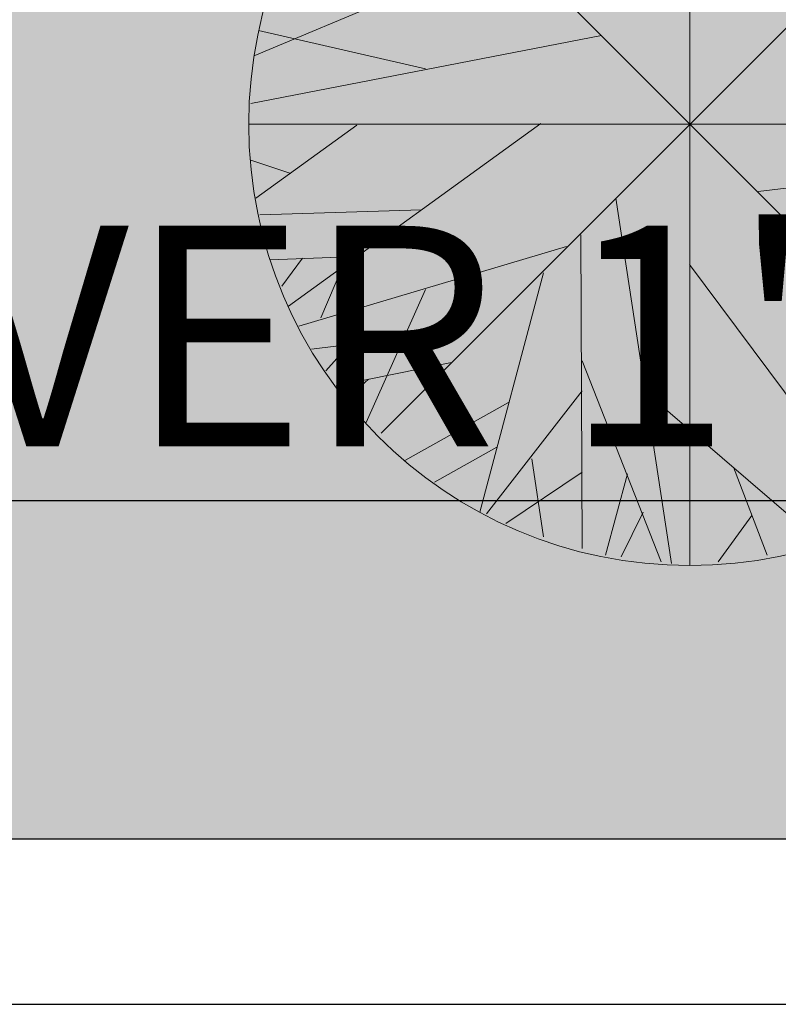
# Model space of a CAD drawing. Units: inches. Extents: x 459864 to 460310, y 324185 to 324787.
# Tile 56 of 112: x 460169 to 460189, y 324195 to 324222. Entities that reach past the tile are written whole.
import ezdxf

# ---------------------------------------------------------------- set-up
doc = ezdxf.new("R2010")
doc.units = ezdxf.units.IN
for name, color, linetype, lineweight in [('A-ANNO-DIMS', 2, 'Continuous', 18), ('C-PROP', 7, 'Continuous', 30), ('L-PLNT', 3, 'Continuous', 13), ('L-SITE-PATT', 252, 'Continuous', 13)]:
    doc.layers.add(name, color=color, linetype=linetype, lineweight=lineweight)
doc.styles.get("Standard").update_dxf_attribs({"font": 'arial.ttf'})
doc.dimstyles.new('ISO-25', dxfattribs={"dimtxt": 6, "dimasz": 2.5, "dimexe": 1.25, "dimexo": 0.625, "dimtad": 1, "dimdec": 1, "dimlunit": 3, "dimtxsty": 'Standard', "dimcen": 2.5, "dimadec": 0, "dimazin": 0, "dimtfac": 1, "dimtdec": 1, "dimtmove": 0, "dimatfit": 3, "dimfxl": 1, "dimarcsym": 0})

# ---------------------------------------------------------------- blocks, each defined once
blk = doc.blocks.new('Tree - deciduous plan')
for p, q in [((0, 59.9996), (0, -60)), ((42, 42), (-42, -42)), ((42, -42), (-42, 42)), ((-32.2571, 20.6333), (-59.1937, 9.348)), ((-59.7219, 2.8025), (-12.0106, 12.0565)), ((-58.6656, 12.7336), (-35.9543, 7.5424)), ((-54.6162, -24.7335), (-20.2853, 0.0941)), ((-60, 0), (60, 0)), ((-45.2853, -0.1316), (-59.0177, -10.0627)), ((9.2922, -9.1598), (59.6443, -2.8401)), ((-59.7219, -4.8714), (-54.2641, -6.6771)), ((-10.074, -10.0627), (-2.5036, -59.7178)), ((-58.4895, -12.3197), (-36.4825, -11.6426)), ((-14.8275, -15.0282), (-14.6515, -57.6865)), ((-53.2078, -27.442), (-16.7641, -16.6081)), ((-57.081, -18.4138), (-45.2853, -17.9624)), ((-52.6797, -18.188), (-55.4966, -22.0251)), ((-47.2219, -19.3166), (-50.2148, -26.3135)), ((-0.0388, -19.0909), (25.8415, -53.8495)), ((-19.9331, -20.2194), (-28.5599, -52.721)), ((-35.9543, -22.4765), (-44.0529, -40.5329)), ((-38.9472, -29.0219), (-51.4472, -30.6018)), ((-46.5177, -30.1504), (-49.5106, -33.536)), ((-32.4331, -32.4075), (-48.1021, -35.5674)), ((-14.6515, -32.1818), (-3.912, -59.4922)), ((-43.7008, -34.6645), (-46.6937, -37.373)), ((-14.6515, -36.2445), (-27.6797, -52.9467)), ((-6.2008, -36.2445), (17.919, -57.0094)), ((-24.6867, -37.8244), (-38.7712, -45.7241)), ((-26.2712, -43.9185), (-34.7219, -48.6583)), ((-21.5177, -45.4984), (-19.9331, -56.1065)), ((5.9471, -46.6269), (10.5246, -58.5893)), ((-14.6515, -47.3041), (-25.0388, -54.3009)), ((-8.4895, -47.5298), (-11.4825, -58.5893)), ((-6.3768, -52.721), (-9.3698, -58.815)), ((8.4119, -53.1724), (3.8344, -59.4922))]:
    blk.add_line(p, q)
blk.add_circle((0, 0), 60)
blk = doc.blocks.new('*D34')
at = {"layer": 'A-ANNO-DIMS', "color": 0, "lineweight": -2, "transparency": 16777216}
for p, q in [((460132.814, 324211.063), (460132.814, 324207.434)), ((460152.838, 324211.063), (460152.838, 324207.434)), ((460135.314, 324208.684), (460150.338, 324208.684)), ((460152.838, 324208.684), (460202.984, 324208.684))]:
    blk.add_line(p, q, dxfattribs=at)
at = {"layer": 'A-ANNO-DIMS', "color": 0, "transparency": 16777216}
for points in [[(460135.314, 324209.101), (460135.314, 324208.268), (460132.814, 324208.684)], [(460150.338, 324209.101), (460150.338, 324208.268), (460152.838, 324208.684)]]:
    blk.add_solid(points, dxfattribs=at)
at = {"layer": 'Defpoints', "color": 0, "transparency": 16777216}
for p in [(460132.814, 324211.688), (460152.838, 324211.688), (460152.838, 324208.684)]:
    blk.add_point(p, dxfattribs=at)
at = {"layer": 'A-ANNO-DIMS', "color": 0, "transparency": 16777216, "insert": (460179.161, 324212.373), "char_height": 6, "attachment_point": 5}
blk.add_mtext('PAVER 1\'-8"', dxfattribs=at)

msp = doc.modelspace()

# ---------------------------------------------------------------- hatches: boundary and pattern name
at = {"layer": 'L-SITE-PATT'}
h = msp.add_hatch(dxfattribs=at)
h.set_pattern_fill('DOTS', color=256)
h.paths.add_polyline_path([(460269.804, 324283.483), (460247.115, 324283.483), (460121.929, 324283.483), (460121.929, 324252.473), (460117.429, 324252.473), (460110.124, 324252.473), (460110.124, 324243.287), (460080.83, 324243.287), (460080.83, 324252.473), (460061.115, 324252.473), (460061.115, 324251.882), (460077.909, 324251.882), (460077.909, 324199.483), (460080.83, 324199.483), (460080.83, 324207.553), (460110.124, 324207.553), (460110.124, 324199.483), (460110.813, 324199.483), (460262.115, 324199.483), (460269.804, 324199.483)], flags=17)
edge = h.paths.add_edge_path(flags=0)
edge.add_ellipse((460222.59, 324263.813), major_axis=(-8.485, 8.485), ratio=1, start_angle=405, end_angle=495, ccw=False)
edge.add_line((460214.821, 324254.66), (460214.832, 324254.666))
edge.add_ellipse((460222.59, 324263.813), major_axis=(-8.485, 8.485), ratio=1, start_angle=405, end_angle=495, ccw=False)
edge.add_line((460210.759, 324261.781), (460210.768, 324261.787))
edge.add_ellipse((460222.59, 324263.813), major_axis=(-8.485, 8.485), ratio=1, start_angle=405, end_angle=495, ccw=False)
edge.add_ellipse((460222.59, 324263.813), major_axis=(-8.485, 8.485), ratio=1, start_angle=392.754, end_angle=405, ccw=False)
edge.add_ellipse((460222.59, 324263.813), major_axis=(-8.485, 8.485), ratio=1, start_angle=380.9347, end_angle=392.754, ccw=False)
edge.add_line((460211.337, 324267.985), (460211.34, 324267.985))
edge.add_ellipse((460222.59, 324263.813), major_axis=(-8.485, 8.485), ratio=1, start_angle=380.9347, end_angle=392.754, ccw=False)
edge.add_ellipse((460222.59, 324263.813), major_axis=(-8.485, 8.485), ratio=1, start_angle=347.9015, end_angle=380.9347, ccw=False)
edge.add_ellipse((460222.59, 324263.813), major_axis=(-8.485, 8.485), ratio=1, start_angle=327.0619, end_angle=347.9015, ccw=False)
edge.add_ellipse((460222.59, 324263.813), major_axis=(-8.485, 8.485), ratio=1, start_angle=278.3246, end_angle=327.0619, ccw=False)
edge.add_line((460225.158, 324275.536), (460225.158, 324275.535))
edge.add_ellipse((460222.59, 324263.813), major_axis=(-8.485, 8.485), ratio=1, start_angle=278.3246, end_angle=327.0619, ccw=False)
edge.add_ellipse((460222.59, 324263.813), major_axis=(-8.485, 8.485), ratio=1, start_angle=260.6436, end_angle=278.3246, ccw=False)
edge.add_ellipse((460222.59, 324263.813), major_axis=(-8.485, 8.485), ratio=1, start_angle=225, end_angle=260.6436, ccw=False)
edge.add_line((460234.509, 324265.243), (460234.501, 324265.239))
edge.add_ellipse((460222.59, 324263.813), major_axis=(-8.485, 8.485), ratio=1, start_angle=225, end_angle=260.6436, ccw=False)
edge.add_ellipse((460222.59, 324263.813), major_axis=(-8.485, 8.485), ratio=1, start_angle=495, end_angle=585, ccw=False)
edge.add_line((460234.437, 324261.861), (460234.424, 324261.858))
edge.add_ellipse((460222.59, 324263.813), major_axis=(-8.485, 8.485), ratio=1, start_angle=495, end_angle=585, ccw=False)
edge.add_line((460227.95, 324253.067), (460227.946, 324253.083))
edge.add_ellipse((460222.59, 324263.813), major_axis=(-8.485, 8.485), ratio=1, start_angle=495, end_angle=585, ccw=False)
edge.add_line((460226.223, 324252.369), (460226.211, 324252.38))
edge.add_ellipse((460222.59, 324263.813), major_axis=(-8.485, 8.485), ratio=1, start_angle=495, end_angle=585, ccw=False)
h.paths.add_polyline_path([(460219.651, 324254.347), (460218.461, 324253.545), (460218.275, 324254.789), (460219.642, 324256.542), (460219.625, 324260.848), (460216.11, 324257.333), (460214.35, 324256.978), (460215.416, 324259.356), (460212.524, 324258.496), (460213.137, 324259.93), (460218.507, 324263.813), (460222.59, 324263.813), (460222.59, 324267.807), (460218.176, 324272.212), (460219.026, 324274.639), (460222.59, 324272.811), (460222.59, 324275.423), (460223.057, 324274.825), (460222.675, 324273.492), (460225.912, 324267.135), (460219.625, 324260.848)], flags=0)
edge = h.paths.add_edge_path(flags=0)
edge.add_ellipse((460194.576, 324264.046), major_axis=(-8.485, 8.485), ratio=1, start_angle=495, end_angle=585, ccw=False)
edge.add_line((460199.936, 324253.3), (460199.932, 324253.316))
edge.add_ellipse((460194.576, 324264.046), major_axis=(-8.485, 8.485), ratio=1, start_angle=495, end_angle=585, ccw=False)
edge.add_line((460198.208, 324252.603), (460198.196, 324252.613))
edge.add_ellipse((460194.576, 324264.046), major_axis=(-8.485, 8.485), ratio=1, start_angle=495, end_angle=585, ccw=False)
edge.add_ellipse((460194.576, 324264.046), major_axis=(-8.485, 8.485), ratio=1, start_angle=405, end_angle=495, ccw=False)
edge.add_line((460186.806, 324254.893), (460186.817, 324254.899))
edge.add_ellipse((460194.576, 324264.046), major_axis=(-8.485, 8.485), ratio=1, start_angle=405, end_angle=495, ccw=False)
edge.add_line((460182.744, 324262.014), (460182.753, 324262.02))
edge.add_ellipse((460194.576, 324264.046), major_axis=(-8.485, 8.485), ratio=1, start_angle=405, end_angle=495, ccw=False)
edge.add_ellipse((460194.576, 324264.046), major_axis=(-8.485, 8.485), ratio=1, start_angle=392.754, end_angle=405, ccw=False)
edge.add_ellipse((460194.576, 324264.046), major_axis=(-8.485, 8.485), ratio=1, start_angle=380.9347, end_angle=392.754, ccw=False)
edge.add_line((460183.323, 324268.218), (460183.326, 324268.218))
edge.add_ellipse((460194.576, 324264.046), major_axis=(-8.485, 8.485), ratio=1, start_angle=380.9347, end_angle=392.754, ccw=False)
edge.add_ellipse((460194.576, 324264.046), major_axis=(-8.485, 8.485), ratio=1, start_angle=347.9015, end_angle=380.9347, ccw=False)
edge.add_ellipse((460194.576, 324264.046), major_axis=(-8.485, 8.485), ratio=1, start_angle=327.0619, end_angle=347.9015, ccw=False)
edge.add_ellipse((460194.576, 324264.046), major_axis=(-8.485, 8.485), ratio=1, start_angle=278.3246, end_angle=327.0619, ccw=False)
edge.add_line((460197.144, 324275.769), (460197.143, 324275.768))
edge.add_ellipse((460194.576, 324264.046), major_axis=(-8.485, 8.485), ratio=1, start_angle=278.3246, end_angle=327.0619, ccw=False)
edge.add_ellipse((460194.576, 324264.046), major_axis=(-8.485, 8.485), ratio=1, start_angle=260.6436, end_angle=278.3246, ccw=False)
edge.add_ellipse((460194.576, 324264.046), major_axis=(-8.485, 8.485), ratio=1, start_angle=225, end_angle=260.6436, ccw=False)
edge.add_line((460206.494, 324265.476), (460206.487, 324265.473))
edge.add_ellipse((460194.576, 324264.046), major_axis=(-8.485, 8.485), ratio=1, start_angle=225, end_angle=260.6436, ccw=False)
edge.add_ellipse((460194.576, 324264.046), major_axis=(-8.485, 8.485), ratio=1, start_angle=495, end_angle=585, ccw=False)
edge.add_line((460206.422, 324262.094), (460206.409, 324262.091))
h.paths.add_polyline_path([(460191.61, 324261.081), (460191.637, 324254.58), (460190.447, 324253.778), (460190.261, 324255.023), (460191.628, 324256.775), (460191.61, 324261.081), (460188.096, 324257.566), (460186.335, 324257.211), (460187.402, 324259.589), (460184.509, 324258.729), (460185.123, 324260.163), (460190.493, 324264.046), (460194.576, 324264.046), (460194.576, 324268.04), (460190.161, 324272.446), (460191.011, 324274.872), (460194.576, 324273.044), (460194.576, 324275.657), (460195.043, 324275.058), (460194.661, 324273.725), (460197.897, 324267.368)], flags=0)
edge = h.paths.add_edge_path(flags=0)
edge.add_ellipse((460252.912, 324263.578), major_axis=(-8.485, 8.485), ratio=1, start_angle=405, end_angle=495, ccw=False)
edge.add_line((460241.081, 324261.545), (460241.089, 324261.551))
edge.add_ellipse((460252.912, 324263.578), major_axis=(-8.485, 8.485), ratio=1, start_angle=405, end_angle=495, ccw=False)
edge.add_ellipse((460252.912, 324263.578), major_axis=(-8.485, 8.485), ratio=1, start_angle=392.754, end_angle=405, ccw=False)
edge.add_ellipse((460252.912, 324263.578), major_axis=(-8.485, 8.485), ratio=1, start_angle=380.9347, end_angle=392.754, ccw=False)
edge.add_line((460241.659, 324267.749), (460241.662, 324267.749))
edge.add_ellipse((460252.912, 324263.578), major_axis=(-8.485, 8.485), ratio=1, start_angle=380.9347, end_angle=392.754, ccw=False)
edge.add_ellipse((460252.912, 324263.578), major_axis=(-8.485, 8.485), ratio=1, start_angle=347.9015, end_angle=380.9347, ccw=False)
edge.add_ellipse((460252.912, 324263.578), major_axis=(-8.485, 8.485), ratio=1, start_angle=327.0619, end_angle=347.9015, ccw=False)
edge.add_ellipse((460252.912, 324263.578), major_axis=(-8.485, 8.485), ratio=1, start_angle=278.3246, end_angle=327.0619, ccw=False)
edge.add_line((460255.48, 324275.3), (460255.479, 324275.299))
edge.add_ellipse((460252.912, 324263.578), major_axis=(-8.485, 8.485), ratio=1, start_angle=278.3246, end_angle=327.0619, ccw=False)
edge.add_ellipse((460252.912, 324263.578), major_axis=(-8.485, 8.485), ratio=1, start_angle=260.6436, end_angle=278.3246, ccw=False)
edge.add_ellipse((460252.912, 324263.578), major_axis=(-8.485, 8.485), ratio=1, start_angle=225, end_angle=260.6436, ccw=False)
edge.add_line((460264.83, 324265.007), (460264.823, 324265.004))
edge.add_ellipse((460252.912, 324263.578), major_axis=(-8.485, 8.485), ratio=1, start_angle=225, end_angle=260.6436, ccw=False)
edge.add_ellipse((460252.912, 324263.578), major_axis=(-8.485, 8.485), ratio=1, start_angle=495, end_angle=585, ccw=False)
edge.add_line((460264.758, 324261.626), (460264.745, 324261.622))
edge.add_ellipse((460252.912, 324263.578), major_axis=(-8.485, 8.485), ratio=1, start_angle=495, end_angle=585, ccw=False)
edge.add_line((460258.272, 324252.832), (460258.268, 324252.848))
edge.add_ellipse((460252.912, 324263.578), major_axis=(-8.485, 8.485), ratio=1, start_angle=495, end_angle=585, ccw=False)
edge.add_line((460256.545, 324252.134), (460256.533, 324252.144))
edge.add_ellipse((460252.912, 324263.578), major_axis=(-8.485, 8.485), ratio=1, start_angle=495, end_angle=585, ccw=False)
edge.add_ellipse((460252.912, 324263.578), major_axis=(-8.485, 8.485), ratio=1, start_angle=405, end_angle=495, ccw=False)
edge.add_line((460245.143, 324254.424), (460245.153, 324254.43))
h.paths.add_polyline_path([(460244.672, 324256.742), (460245.738, 324259.12), (460242.846, 324258.26), (460243.459, 324259.694), (460248.829, 324263.578), (460252.912, 324263.578), (460252.912, 324267.571), (460248.497, 324271.977), (460249.348, 324274.403), (460252.912, 324272.576), (460252.912, 324275.188), (460253.379, 324274.589), (460252.997, 324273.257), (460256.233, 324266.899), (460249.946, 324260.612), (460249.973, 324254.111), (460248.783, 324253.309), (460248.597, 324254.554), (460249.964, 324256.306), (460249.946, 324260.612), (460246.432, 324257.097)], flags=0)
edge = h.paths.add_edge_path(flags=0)
edge.add_ellipse((460167.439, 324262.833), major_axis=(-8.485, 8.485), ratio=1, start_angle=495, end_angle=585, ccw=False)
edge.add_line((460172.799, 324252.087), (460172.795, 324252.103))
edge.add_ellipse((460167.439, 324262.833), major_axis=(-8.485, 8.485), ratio=1, start_angle=495, end_angle=585, ccw=False)
edge.add_line((460171.071, 324251.389), (460171.059, 324251.399))
edge.add_ellipse((460167.439, 324262.833), major_axis=(-8.485, 8.485), ratio=1, start_angle=495, end_angle=585, ccw=False)
edge.add_ellipse((460167.439, 324262.833), major_axis=(-8.485, 8.485), ratio=1, start_angle=405, end_angle=495, ccw=False)
edge.add_line((460159.669, 324253.679), (460159.68, 324253.685))
edge.add_ellipse((460167.439, 324262.833), major_axis=(-8.485, 8.485), ratio=1, start_angle=405, end_angle=495, ccw=False)
edge.add_line((460155.607, 324260.8), (460155.616, 324260.806))
edge.add_ellipse((460167.439, 324262.833), major_axis=(-8.485, 8.485), ratio=1, start_angle=405, end_angle=495, ccw=False)
edge.add_ellipse((460167.439, 324262.833), major_axis=(-8.485, 8.485), ratio=1, start_angle=392.754, end_angle=405, ccw=False)
edge.add_ellipse((460167.439, 324262.833), major_axis=(-8.485, 8.485), ratio=1, start_angle=380.9347, end_angle=392.754, ccw=False)
edge.add_line((460156.185, 324267.005), (460156.189, 324267.005))
edge.add_ellipse((460167.439, 324262.833), major_axis=(-8.485, 8.485), ratio=1, start_angle=380.9347, end_angle=392.754, ccw=False)
edge.add_ellipse((460167.439, 324262.833), major_axis=(-8.485, 8.485), ratio=1, start_angle=347.9015, end_angle=380.9347, ccw=False)
edge.add_ellipse((460167.439, 324262.833), major_axis=(-8.485, 8.485), ratio=1, start_angle=327.0619, end_angle=347.9015, ccw=False)
edge.add_ellipse((460167.439, 324262.833), major_axis=(-8.485, 8.485), ratio=1, start_angle=278.3246, end_angle=327.0619, ccw=False)
edge.add_line((460170.007, 324274.556), (460170.006, 324274.554))
edge.add_ellipse((460167.439, 324262.833), major_axis=(-8.485, 8.485), ratio=1, start_angle=278.3246, end_angle=327.0619, ccw=False)
edge.add_ellipse((460167.439, 324262.833), major_axis=(-8.485, 8.485), ratio=1, start_angle=260.6436, end_angle=278.3246, ccw=False)
edge.add_ellipse((460167.439, 324262.833), major_axis=(-8.485, 8.485), ratio=1, start_angle=225, end_angle=260.6436, ccw=False)
edge.add_line((460179.357, 324264.262), (460179.35, 324264.259))
edge.add_ellipse((460167.439, 324262.833), major_axis=(-8.485, 8.485), ratio=1, start_angle=225, end_angle=260.6436, ccw=False)
edge.add_ellipse((460167.439, 324262.833), major_axis=(-8.485, 8.485), ratio=1, start_angle=495, end_angle=585, ccw=False)
edge.add_line((460179.285, 324260.881), (460179.272, 324260.877))
h.paths.add_polyline_path([(460164.473, 324259.867), (460164.5, 324253.366), (460163.31, 324252.565), (460163.124, 324253.809), (460164.491, 324255.561), (460164.473, 324259.867), (460160.958, 324256.353), (460159.198, 324255.998), (460160.265, 324258.375), (460157.372, 324257.515), (460157.986, 324258.949), (460163.356, 324262.833), (460167.439, 324262.833), (460167.439, 324266.826), (460163.024, 324271.232), (460163.874, 324273.659), (460167.439, 324271.831), (460167.439, 324274.443), (460167.905, 324273.844), (460167.524, 324272.512), (460170.76, 324266.154)], flags=0)
edge = h.paths.add_edge_path(flags=0)
edge.add_ellipse((460140.758, 324262.37), major_axis=(-8.485, 8.485), ratio=1, start_angle=495, end_angle=585, ccw=False)
edge.add_line((460146.118, 324251.624), (460146.114, 324251.639))
edge.add_ellipse((460140.758, 324262.37), major_axis=(-8.485, 8.485), ratio=1, start_angle=495, end_angle=585, ccw=False)
edge.add_line((460144.391, 324250.926), (460144.379, 324250.936))
edge.add_ellipse((460140.758, 324262.37), major_axis=(-8.485, 8.485), ratio=1, start_angle=495, end_angle=585, ccw=False)
edge.add_ellipse((460140.758, 324262.37), major_axis=(-8.485, 8.485), ratio=1, start_angle=405, end_angle=495, ccw=False)
edge.add_line((460132.989, 324253.216), (460132.999, 324253.222))
edge.add_ellipse((460140.758, 324262.37), major_axis=(-8.485, 8.485), ratio=1, start_angle=405, end_angle=495, ccw=False)
edge.add_line((460128.927, 324260.337), (460128.935, 324260.343))
edge.add_ellipse((460140.758, 324262.37), major_axis=(-8.485, 8.485), ratio=1, start_angle=405, end_angle=495, ccw=False)
edge.add_ellipse((460140.758, 324262.37), major_axis=(-8.485, 8.485), ratio=1, start_angle=392.754, end_angle=405, ccw=False)
edge.add_ellipse((460140.758, 324262.37), major_axis=(-8.485, 8.485), ratio=1, start_angle=380.9347, end_angle=392.754, ccw=False)
edge.add_line((460129.505, 324266.541), (460129.508, 324266.541))
edge.add_ellipse((460140.758, 324262.37), major_axis=(-8.485, 8.485), ratio=1, start_angle=380.9347, end_angle=392.754, ccw=False)
edge.add_ellipse((460140.758, 324262.37), major_axis=(-8.485, 8.485), ratio=1, start_angle=347.9015, end_angle=380.9347, ccw=False)
edge.add_ellipse((460140.758, 324262.37), major_axis=(-8.485, 8.485), ratio=1, start_angle=327.0619, end_angle=347.9015, ccw=False)
edge.add_ellipse((460140.758, 324262.37), major_axis=(-8.485, 8.485), ratio=1, start_angle=278.3246, end_angle=327.0619, ccw=False)
edge.add_line((460143.326, 324274.092), (460143.325, 324274.091))
edge.add_ellipse((460140.758, 324262.37), major_axis=(-8.485, 8.485), ratio=1, start_angle=278.3246, end_angle=327.0619, ccw=False)
edge.add_ellipse((460140.758, 324262.37), major_axis=(-8.485, 8.485), ratio=1, start_angle=260.6436, end_angle=278.3246, ccw=False)
edge.add_ellipse((460140.758, 324262.37), major_axis=(-8.485, 8.485), ratio=1, start_angle=225, end_angle=260.6436, ccw=False)
edge.add_line((460152.677, 324263.799), (460152.669, 324263.796))
edge.add_ellipse((460140.758, 324262.37), major_axis=(-8.485, 8.485), ratio=1, start_angle=225, end_angle=260.6436, ccw=False)
edge.add_ellipse((460140.758, 324262.37), major_axis=(-8.485, 8.485), ratio=1, start_angle=495, end_angle=585, ccw=False)
edge.add_line((460152.604, 324260.418), (460152.592, 324260.414))
h.paths.add_polyline_path([(460137.792, 324259.404), (460137.819, 324252.903), (460136.629, 324252.101), (460136.443, 324253.346), (460137.81, 324255.098), (460137.792, 324259.404), (460134.278, 324255.889), (460132.518, 324255.534), (460133.584, 324257.912), (460130.692, 324257.052), (460131.305, 324258.486), (460136.675, 324262.37), (460140.758, 324262.37), (460140.758, 324266.363), (460136.343, 324270.769), (460137.194, 324273.195), (460140.758, 324271.367), (460140.758, 324273.98), (460141.225, 324273.381), (460140.843, 324272.049), (460144.079, 324265.691)], flags=0)
h.paths.add_polyline_path([(460110.124, 324227.414), (460080.83, 324227.414), (460080.83, 324235.484), (460110.124, 324235.484)], flags=16)
h.paths.add_polyline_path([(460110.124, 324220.797), (460110.124, 324212.727), (460080.83, 324212.727), (460080.83, 324220.797)], flags=16)
h.paths.add_polyline_path([(460269.804, 324283.483), (460247.115, 324283.483), (460121.929, 324283.483), (460121.929, 324252.473), (460117.429, 324252.473), (460110.124, 324252.473), (460110.124, 324243.287), (460080.83, 324243.287), (460080.83, 324252.473), (460061.115, 324252.473), (460061.115, 324251.882), (460077.909, 324251.882), (460077.909, 324199.483), (460080.83, 324199.483), (460080.83, 324207.553), (460110.124, 324207.553), (460110.124, 324199.483), (460262.115, 324199.483), (460269.804, 324199.483)], flags=17)
h.paths.add_polyline_path([(460219.651, 324254.347), (460218.461, 324253.545), (460218.275, 324254.789), (460219.642, 324256.542), (460219.625, 324260.848), (460216.11, 324257.333), (460214.35, 324256.978), (460215.416, 324259.356), (460212.524, 324258.496), (460213.137, 324259.93), (460218.507, 324263.813), (460222.59, 324263.813), (460220.18, 324266.223), (460215.461, 324265.308), (460211.835, 324266.137), (460216.247, 324267.985), (460218.418, 324267.985), (460222.59, 324263.813), (460222.59, 324267.807), (460218.176, 324272.212), (460219.026, 324274.639), (460222.59, 324272.811), (460222.59, 324275.423), (460223.057, 324274.825), (460222.675, 324273.492), (460225.912, 324267.135), (460222.59, 324263.813), (460231.383, 324263.813), (460228.485, 324262.488), (460224.425, 324261.978), (460228.68, 324257.724), (460228.966, 324254.791), (460227.142, 324256.537), (460227.542, 324254.819), (460227.333, 324253.614), (460222.59, 324259.985), (460222.59, 324255.497), (460221.377, 324256.541), (460220.576, 324261.799), (460219.625, 324260.848)], flags=0)
h.paths.add_polyline_path([(460199.127, 324256.77), (460199.528, 324255.052), (460199.319, 324253.848), (460194.576, 324260.218), (460194.576, 324255.73), (460193.363, 324256.774), (460192.561, 324262.032), (460191.61, 324261.081), (460191.637, 324254.58), (460190.447, 324253.778), (460190.261, 324255.023), (460191.628, 324256.775), (460191.61, 324261.081), (460188.096, 324257.566), (460186.335, 324257.211), (460187.402, 324259.589), (460184.509, 324258.729), (460185.123, 324260.163), (460190.493, 324264.046), (460194.576, 324264.046), (460192.166, 324266.456), (460187.446, 324265.541), (460183.82, 324266.37), (460188.232, 324268.218), (460190.404, 324268.218), (460194.576, 324264.046), (460194.576, 324268.04), (460190.161, 324272.446), (460191.011, 324274.872), (460194.576, 324273.044), (460194.576, 324275.657), (460195.043, 324275.058), (460194.661, 324273.725), (460197.897, 324267.368), (460194.576, 324264.046), (460203.368, 324264.046), (460200.47, 324262.721), (460196.411, 324262.212), (460200.665, 324257.957), (460200.951, 324255.024)], flags=0)
h.paths.add_polyline_path([(460244.672, 324256.742), (460245.738, 324259.12), (460242.846, 324258.26), (460243.459, 324259.694), (460248.829, 324263.578), (460252.912, 324263.578), (460250.502, 324265.987), (460245.783, 324265.072), (460242.156, 324265.901), (460246.568, 324267.749), (460248.74, 324267.749), (460252.912, 324263.578), (460252.912, 324267.571), (460248.497, 324271.977), (460249.348, 324274.403), (460252.912, 324272.576), (460252.912, 324275.188), (460253.379, 324274.589), (460252.997, 324273.257), (460256.233, 324266.899), (460252.912, 324263.578), (460261.705, 324263.578), (460258.806, 324262.252), (460254.747, 324261.743), (460259.002, 324257.488), (460259.288, 324254.555), (460257.463, 324256.301), (460257.864, 324254.583), (460257.655, 324253.379), (460252.912, 324259.749), (460252.912, 324255.261), (460251.699, 324256.305), (460250.897, 324261.563), (460249.946, 324260.612), (460249.973, 324254.111), (460248.783, 324253.309), (460248.597, 324254.554), (460249.964, 324256.306), (460249.946, 324260.612), (460246.432, 324257.097)], flags=0)
h.paths.add_polyline_path([(460173.528, 324256.743), (460173.814, 324253.811), (460171.99, 324255.556), (460172.39, 324253.838), (460172.182, 324252.634), (460167.439, 324259.004), (460167.439, 324254.516), (460166.226, 324255.56), (460165.424, 324260.818), (460164.473, 324259.867), (460164.5, 324253.366), (460163.31, 324252.565), (460163.124, 324253.809), (460164.491, 324255.561), (460164.473, 324259.867), (460160.958, 324256.353), (460159.198, 324255.998), (460160.265, 324258.375), (460157.372, 324257.515), (460157.986, 324258.949), (460163.356, 324262.833), (460167.439, 324262.833), (460165.029, 324265.243), (460160.309, 324264.327), (460156.683, 324265.156), (460161.095, 324267.005), (460163.267, 324267.005), (460167.439, 324262.833), (460167.439, 324266.826), (460163.024, 324271.232), (460163.874, 324273.659), (460167.439, 324271.831), (460167.439, 324274.443), (460167.905, 324273.844), (460167.524, 324272.512), (460170.76, 324266.154), (460167.439, 324262.833), (460176.231, 324262.833), (460173.333, 324261.507), (460169.274, 324260.998)], flags=0)
h.paths.add_polyline_path([(460146.848, 324256.28), (460147.134, 324253.347), (460145.31, 324255.093), (460145.71, 324253.375), (460145.501, 324252.171), (460140.758, 324258.541), (460140.758, 324254.053), (460139.545, 324255.097), (460138.744, 324260.355), (460137.792, 324259.404), (460137.819, 324252.903), (460136.629, 324252.101), (460136.443, 324253.346), (460137.81, 324255.098), (460137.792, 324259.404), (460134.278, 324255.889), (460132.518, 324255.534), (460133.584, 324257.912), (460130.692, 324257.052), (460131.305, 324258.486), (460136.675, 324262.37), (460140.758, 324262.37), (460138.348, 324264.779), (460133.629, 324263.864), (460130.002, 324264.693), (460134.414, 324266.541), (460136.586, 324266.541), (460140.758, 324262.37), (460140.758, 324266.363), (460136.343, 324270.769), (460137.194, 324273.195), (460140.758, 324271.367), (460140.758, 324273.98), (460141.225, 324273.381), (460140.843, 324272.049), (460144.079, 324265.691), (460140.758, 324262.37), (460149.551, 324262.37), (460146.653, 324261.044), (460142.593, 324260.535)], flags=0)
edge = h.paths.add_edge_path()
edge.add_line((460269.804, 324272.549), (460260.881, 324272.549))
edge.add_ellipse((460252.912, 324263.578), major_axis=(-8.485, 8.485), ratio=1, start_angle=260.6436, end_angle=273.3846, ccw=False)
edge.add_line((460262.283, 324271.092), (460262.261, 324271.091))
edge.add_ellipse((460252.912, 324263.578), major_axis=(-8.485, 8.485), ratio=1, start_angle=260.6436, end_angle=273.3846, ccw=False)
edge.add_ellipse((460252.912, 324263.578), major_axis=(-8.485, 8.485), ratio=1, start_angle=225, end_angle=260.6436, ccw=False)
edge.add_line((460263.609, 324269.063), (460263.572, 324269.058))
edge.add_ellipse((460252.912, 324263.578), major_axis=(-8.485, 8.485), ratio=1, start_angle=225, end_angle=260.6436, ccw=False)
edge.add_line((460264.615, 324266.306), (460264.585, 324266.305))
edge.add_ellipse((460252.912, 324263.578), major_axis=(-8.485, 8.485), ratio=1, start_angle=225, end_angle=260.6436, ccw=False)
edge.add_line((460264.83, 324265.007), (460264.823, 324265.004))
edge.add_ellipse((460252.912, 324263.578), major_axis=(-8.485, 8.485), ratio=1, start_angle=225, end_angle=260.6436, ccw=False)
edge.add_ellipse((460252.912, 324263.578), major_axis=(-8.485, 8.485), ratio=1, start_angle=495, end_angle=585, ccw=False)
edge.add_line((460264.758, 324261.626), (460264.745, 324261.622))
edge.add_ellipse((460252.912, 324263.578), major_axis=(-8.485, 8.485), ratio=1, start_angle=495, end_angle=585, ccw=False)
edge.add_line((460263.442, 324257.739), (460263.389, 324257.779))
edge.add_ellipse((460252.912, 324263.578), major_axis=(-8.485, 8.485), ratio=1, start_angle=495, end_angle=585, ccw=False)
edge.add_line((460258.128, 324252.744), (460258.102, 324252.779))
edge.add_ellipse((460252.912, 324263.578), major_axis=(-8.485, 8.485), ratio=1, start_angle=495, end_angle=585, ccw=False)
edge.add_line((460256.545, 324252.134), (460256.533, 324252.144))
edge.add_ellipse((460252.912, 324263.578), major_axis=(-8.485, 8.485), ratio=1, start_angle=495, end_angle=585, ccw=False)
edge.add_ellipse((460252.912, 324263.578), major_axis=(-8.485, 8.485), ratio=1, start_angle=405, end_angle=495, ccw=False)
edge.add_line((460250.594, 324251.78), (460250.605, 324251.82))
edge.add_ellipse((460252.912, 324263.578), major_axis=(-8.485, 8.485), ratio=1, start_angle=405, end_angle=495, ccw=False)
edge.add_line((460245.143, 324254.424), (460245.153, 324254.43))
edge.add_ellipse((460252.912, 324263.578), major_axis=(-8.485, 8.485), ratio=1, start_angle=405, end_angle=495, ccw=False)
edge.add_line((460243.525, 324256.059), (460243.56, 324256.091))
edge.add_ellipse((460252.912, 324263.578), major_axis=(-8.485, 8.485), ratio=1, start_angle=405, end_angle=495, ccw=False)
edge.add_line((460241.44, 324259.893), (460241.522, 324259.896))
edge.add_ellipse((460252.912, 324263.578), major_axis=(-8.485, 8.485), ratio=1, start_angle=405, end_angle=495, ccw=False)
edge.add_line((460241.081, 324261.545), (460241.089, 324261.551))
edge.add_ellipse((460252.912, 324263.578), major_axis=(-8.485, 8.485), ratio=1, start_angle=405, end_angle=495, ccw=False)
edge.add_ellipse((460252.912, 324263.578), major_axis=(-8.485, 8.485), ratio=1, start_angle=392.754, end_angle=405, ccw=False)
edge.add_line((460241.05, 324265.438), (460241.063, 324265.443))
edge.add_ellipse((460252.912, 324263.578), major_axis=(-8.485, 8.485), ratio=1, start_angle=392.754, end_angle=405, ccw=False)
edge.add_ellipse((460252.912, 324263.578), major_axis=(-8.485, 8.485), ratio=1, start_angle=380.9347, end_angle=392.754, ccw=False)
edge.add_line((460241.452, 324267.176), (460241.469, 324267.171))
edge.add_ellipse((460252.912, 324263.578), major_axis=(-8.485, 8.485), ratio=1, start_angle=380.9347, end_angle=392.754, ccw=False)
edge.add_line((460241.659, 324267.749), (460241.662, 324267.749))
edge.add_ellipse((460252.912, 324263.578), major_axis=(-8.485, 8.485), ratio=1, start_angle=380.9347, end_angle=392.754, ccw=False)
edge.add_ellipse((460252.912, 324263.578), major_axis=(-8.485, 8.485), ratio=1, start_angle=356.6154, end_angle=380.9347, ccw=False)
edge.add_line((460244.88, 324272.488), (460244.713, 324272.549))
edge.add_line((460244.713, 324272.549), (460230.817, 324272.549))
edge.add_ellipse((460222.59, 324263.813), major_axis=(-8.485, 8.485), ratio=1, start_angle=260.6436, end_angle=271.7178, ccw=False)
edge.add_ellipse((460222.59, 324263.813), major_axis=(-8.485, 8.485), ratio=1, start_angle=225, end_angle=260.6436, ccw=False)
edge.add_line((460233.287, 324269.299), (460233.25, 324269.294))
edge.add_ellipse((460222.59, 324263.813), major_axis=(-8.485, 8.485), ratio=1, start_angle=225, end_angle=260.6436, ccw=False)
edge.add_line((460234.294, 324266.541), (460234.264, 324266.541))
edge.add_ellipse((460222.59, 324263.813), major_axis=(-8.485, 8.485), ratio=1, start_angle=225, end_angle=260.6436, ccw=False)
edge.add_line((460234.509, 324265.243), (460234.501, 324265.239))
edge.add_ellipse((460222.59, 324263.813), major_axis=(-8.485, 8.485), ratio=1, start_angle=225, end_angle=260.6436, ccw=False)
edge.add_ellipse((460222.59, 324263.813), major_axis=(-8.485, 8.485), ratio=1, start_angle=495, end_angle=585, ccw=False)
edge.add_line((460234.437, 324261.861), (460234.424, 324261.858))
edge.add_ellipse((460222.59, 324263.813), major_axis=(-8.485, 8.485), ratio=1, start_angle=495, end_angle=585, ccw=False)
edge.add_line((460233.121, 324257.975), (460233.068, 324258.015))
edge.add_ellipse((460222.59, 324263.813), major_axis=(-8.485, 8.485), ratio=1, start_angle=495, end_angle=585, ccw=False)
edge.add_line((460227.806, 324252.979), (460227.78, 324253.014))
edge.add_ellipse((460222.59, 324263.813), major_axis=(-8.485, 8.485), ratio=1, start_angle=495, end_angle=585, ccw=False)
edge.add_line((460226.223, 324252.369), (460226.211, 324252.38))
edge.add_ellipse((460222.59, 324263.813), major_axis=(-8.485, 8.485), ratio=1, start_angle=495, end_angle=585, ccw=False)
edge.add_ellipse((460222.59, 324263.813), major_axis=(-8.485, 8.485), ratio=1, start_angle=405, end_angle=495, ccw=False)
edge.add_line((460220.272, 324252.016), (460220.283, 324252.055))
edge.add_ellipse((460222.59, 324263.813), major_axis=(-8.485, 8.485), ratio=1, start_angle=405, end_angle=495, ccw=False)
edge.add_line((460214.821, 324254.66), (460214.832, 324254.666))
edge.add_ellipse((460222.59, 324263.813), major_axis=(-8.485, 8.485), ratio=1, start_angle=405, end_angle=495, ccw=False)
edge.add_line((460213.203, 324256.295), (460213.239, 324256.327))
edge.add_ellipse((460222.59, 324263.813), major_axis=(-8.485, 8.485), ratio=1, start_angle=405, end_angle=495, ccw=False)
edge.add_line((460211.118, 324260.128), (460211.201, 324260.131))
edge.add_ellipse((460222.59, 324263.813), major_axis=(-8.485, 8.485), ratio=1, start_angle=405, end_angle=495, ccw=False)
edge.add_line((460210.759, 324261.781), (460210.768, 324261.787))
edge.add_ellipse((460222.59, 324263.813), major_axis=(-8.485, 8.485), ratio=1, start_angle=405, end_angle=495, ccw=False)
edge.add_ellipse((460222.59, 324263.813), major_axis=(-8.485, 8.485), ratio=1, start_angle=392.754, end_angle=405, ccw=False)
edge.add_line((460210.729, 324265.673), (460210.741, 324265.678))
edge.add_ellipse((460222.59, 324263.813), major_axis=(-8.485, 8.485), ratio=1, start_angle=392.754, end_angle=405, ccw=False)
edge.add_ellipse((460222.59, 324263.813), major_axis=(-8.485, 8.485), ratio=1, start_angle=380.9347, end_angle=392.754, ccw=False)
edge.add_line((460211.13, 324267.412), (460211.147, 324267.407))
edge.add_ellipse((460222.59, 324263.813), major_axis=(-8.485, 8.485), ratio=1, start_angle=380.9347, end_angle=392.754, ccw=False)
edge.add_line((460211.337, 324267.985), (460211.34, 324267.985))
edge.add_ellipse((460222.59, 324263.813), major_axis=(-8.485, 8.485), ratio=1, start_angle=380.9347, end_angle=392.754, ccw=False)
edge.add_ellipse((460222.59, 324263.813), major_axis=(-8.485, 8.485), ratio=1, start_angle=358.2822, end_angle=380.9347, ccw=False)
edge.add_line((460213.705, 324271.902), (460213.709, 324271.869))
edge.add_ellipse((460222.59, 324263.813), major_axis=(-8.485, 8.485), ratio=1, start_angle=358.2822, end_angle=380.9347, ccw=False)
edge.add_line((460214.363, 324272.549), (460203.078, 324272.549))
edge.add_line((460203.078, 324272.549), (460203.06, 324272.531))
edge.add_ellipse((460194.576, 324264.046), major_axis=(-8.485, 8.485), ratio=1, start_angle=260.6436, end_angle=270.1168, ccw=False)
edge.add_line((460203.957, 324271.561), (460203.921, 324271.56))
edge.add_ellipse((460194.576, 324264.046), major_axis=(-8.485, 8.485), ratio=1, start_angle=260.6436, end_angle=270.1168, ccw=False)
edge.add_ellipse((460194.576, 324264.046), major_axis=(-8.485, 8.485), ratio=1, start_angle=225, end_angle=260.6436, ccw=False)
edge.add_line((460205.272, 324269.532), (460205.235, 324269.527))
edge.add_ellipse((460194.576, 324264.046), major_axis=(-8.485, 8.485), ratio=1, start_angle=225, end_angle=260.6436, ccw=False)
edge.add_line((460206.279, 324266.774), (460206.249, 324266.774))
edge.add_ellipse((460194.576, 324264.046), major_axis=(-8.485, 8.485), ratio=1, start_angle=225, end_angle=260.6436, ccw=False)
edge.add_line((460206.494, 324265.476), (460206.487, 324265.473))
edge.add_ellipse((460194.576, 324264.046), major_axis=(-8.485, 8.485), ratio=1, start_angle=225, end_angle=260.6436, ccw=False)
edge.add_ellipse((460194.576, 324264.046), major_axis=(-8.485, 8.485), ratio=1, start_angle=495, end_angle=585, ccw=False)
edge.add_line((460206.422, 324262.094), (460206.409, 324262.091))
edge.add_ellipse((460194.576, 324264.046), major_axis=(-8.485, 8.485), ratio=1, start_angle=495, end_angle=585, ccw=False)
edge.add_line((460205.106, 324258.208), (460205.053, 324258.248))
edge.add_ellipse((460194.576, 324264.046), major_axis=(-8.485, 8.485), ratio=1, start_angle=495, end_angle=585, ccw=False)
edge.add_line((460199.792, 324253.212), (460199.766, 324253.248))
edge.add_ellipse((460194.576, 324264.046), major_axis=(-8.485, 8.485), ratio=1, start_angle=495, end_angle=585, ccw=False)
edge.add_line((460198.208, 324252.603), (460198.196, 324252.613))
edge.add_ellipse((460194.576, 324264.046), major_axis=(-8.485, 8.485), ratio=1, start_angle=495, end_angle=585, ccw=False)
edge.add_ellipse((460194.576, 324264.046), major_axis=(-8.485, 8.485), ratio=1, start_angle=405, end_angle=495, ccw=False)
edge.add_line((460192.258, 324252.249), (460192.268, 324252.289))
edge.add_ellipse((460194.576, 324264.046), major_axis=(-8.485, 8.485), ratio=1, start_angle=405, end_angle=495, ccw=False)
edge.add_line((460186.806, 324254.893), (460186.817, 324254.899))
edge.add_ellipse((460194.576, 324264.046), major_axis=(-8.485, 8.485), ratio=1, start_angle=405, end_angle=495, ccw=False)
edge.add_line((460185.188, 324256.528), (460185.224, 324256.56))
edge.add_ellipse((460194.576, 324264.046), major_axis=(-8.485, 8.485), ratio=1, start_angle=405, end_angle=495, ccw=False)
edge.add_line((460183.104, 324260.362), (460183.186, 324260.365))
edge.add_ellipse((460194.576, 324264.046), major_axis=(-8.485, 8.485), ratio=1, start_angle=405, end_angle=495, ccw=False)
edge.add_line((460182.744, 324262.014), (460182.753, 324262.02))
edge.add_ellipse((460194.576, 324264.046), major_axis=(-8.485, 8.485), ratio=1, start_angle=405, end_angle=495, ccw=False)
edge.add_ellipse((460194.576, 324264.046), major_axis=(-8.485, 8.485), ratio=1, start_angle=392.754, end_angle=405, ccw=False)
edge.add_line((460182.714, 324265.906), (460182.726, 324265.912))
edge.add_ellipse((460194.576, 324264.046), major_axis=(-8.485, 8.485), ratio=1, start_angle=392.754, end_angle=405, ccw=False)
edge.add_ellipse((460194.576, 324264.046), major_axis=(-8.485, 8.485), ratio=1, start_angle=380.9347, end_angle=392.754, ccw=False)
edge.add_line((460183.116, 324267.645), (460183.133, 324267.64))
edge.add_ellipse((460194.576, 324264.046), major_axis=(-8.485, 8.485), ratio=1, start_angle=380.9347, end_angle=392.754, ccw=False)
edge.add_line((460183.323, 324268.218), (460183.326, 324268.218))
edge.add_ellipse((460194.576, 324264.046), major_axis=(-8.485, 8.485), ratio=1, start_angle=380.9347, end_angle=392.754, ccw=False)
edge.add_ellipse((460194.576, 324264.046), major_axis=(-8.485, 8.485), ratio=1, start_angle=359.8832, end_angle=380.9347, ccw=False)
edge.add_line((460184.491, 324270.611), (460184.553, 324270.611))
edge.add_ellipse((460194.576, 324264.046), major_axis=(-8.485, 8.485), ratio=1, start_angle=359.8832, end_angle=380.9347, ccw=False)
edge.add_line((460185.346, 324271.76), (460185.379, 324271.728))
edge.add_ellipse((460194.576, 324264.046), major_axis=(-8.485, 8.485), ratio=1, start_angle=359.8832, end_angle=380.9347, ccw=False)
edge.add_line((460185.697, 324272.086), (460185.633, 324272.549))
edge.add_line((460185.633, 324272.549), (460174.683, 324272.549))
edge.add_line((460174.683, 324272.549), (460174.606, 324272.457))
edge.add_ellipse((460167.439, 324262.833), major_axis=(-8.485, 8.485), ratio=1, start_angle=260.6436, end_angle=278.3246, ccw=False)
edge.add_ellipse((460167.439, 324262.833), major_axis=(-8.485, 8.485), ratio=1, start_angle=225, end_angle=260.6436, ccw=False)
edge.add_line((460178.135, 324268.318), (460178.098, 324268.313))
edge.add_ellipse((460167.439, 324262.833), major_axis=(-8.485, 8.485), ratio=1, start_angle=225, end_angle=260.6436, ccw=False)
edge.add_line((460179.142, 324265.561), (460179.112, 324265.56))
edge.add_ellipse((460167.439, 324262.833), major_axis=(-8.485, 8.485), ratio=1, start_angle=225, end_angle=260.6436, ccw=False)
edge.add_line((460179.357, 324264.262), (460179.35, 324264.259))
edge.add_ellipse((460167.439, 324262.833), major_axis=(-8.485, 8.485), ratio=1, start_angle=225, end_angle=260.6436, ccw=False)
edge.add_ellipse((460167.439, 324262.833), major_axis=(-8.485, 8.485), ratio=1, start_angle=495, end_angle=585, ccw=False)
edge.add_line((460179.285, 324260.881), (460179.272, 324260.877))
edge.add_ellipse((460167.439, 324262.833), major_axis=(-8.485, 8.485), ratio=1, start_angle=495, end_angle=585, ccw=False)
edge.add_line((460177.969, 324256.994), (460177.916, 324257.034))
edge.add_ellipse((460167.439, 324262.833), major_axis=(-8.485, 8.485), ratio=1, start_angle=495, end_angle=585, ccw=False)
edge.add_line((460172.655, 324251.999), (460172.629, 324252.034))
edge.add_ellipse((460167.439, 324262.833), major_axis=(-8.485, 8.485), ratio=1, start_angle=495, end_angle=585, ccw=False)
edge.add_line((460171.071, 324251.389), (460171.059, 324251.399))
edge.add_ellipse((460167.439, 324262.833), major_axis=(-8.485, 8.485), ratio=1, start_angle=495, end_angle=585, ccw=False)
edge.add_ellipse((460167.439, 324262.833), major_axis=(-8.485, 8.485), ratio=1, start_angle=405, end_angle=495, ccw=False)
edge.add_line((460165.121, 324251.036), (460165.131, 324251.075))
edge.add_ellipse((460167.439, 324262.833), major_axis=(-8.485, 8.485), ratio=1, start_angle=405, end_angle=495, ccw=False)
edge.add_line((460159.669, 324253.679), (460159.68, 324253.685))
edge.add_ellipse((460167.439, 324262.833), major_axis=(-8.485, 8.485), ratio=1, start_angle=405, end_angle=495, ccw=False)
edge.add_line((460158.051, 324255.314), (460158.087, 324255.347))
edge.add_ellipse((460167.439, 324262.833), major_axis=(-8.485, 8.485), ratio=1, start_angle=405, end_angle=495, ccw=False)
edge.add_line((460155.967, 324259.148), (460156.049, 324259.151))
edge.add_ellipse((460167.439, 324262.833), major_axis=(-8.485, 8.485), ratio=1, start_angle=405, end_angle=495, ccw=False)
edge.add_line((460155.607, 324260.8), (460155.616, 324260.806))
edge.add_ellipse((460167.439, 324262.833), major_axis=(-8.485, 8.485), ratio=1, start_angle=405, end_angle=495, ccw=False)
edge.add_ellipse((460167.439, 324262.833), major_axis=(-8.485, 8.485), ratio=1, start_angle=392.754, end_angle=405, ccw=False)
edge.add_line((460155.577, 324264.693), (460155.589, 324264.698))
edge.add_ellipse((460167.439, 324262.833), major_axis=(-8.485, 8.485), ratio=1, start_angle=392.754, end_angle=405, ccw=False)
edge.add_ellipse((460167.439, 324262.833), major_axis=(-8.485, 8.485), ratio=1, start_angle=380.9347, end_angle=392.754, ccw=False)
edge.add_line((460155.979, 324266.432), (460155.996, 324266.426))
edge.add_ellipse((460167.439, 324262.833), major_axis=(-8.485, 8.485), ratio=1, start_angle=380.9347, end_angle=392.754, ccw=False)
edge.add_line((460156.185, 324267.005), (460156.189, 324267.005))
edge.add_ellipse((460167.439, 324262.833), major_axis=(-8.485, 8.485), ratio=1, start_angle=380.9347, end_angle=392.754, ccw=False)
edge.add_ellipse((460167.439, 324262.833), major_axis=(-8.485, 8.485), ratio=1, start_angle=350.9345, end_angle=380.9347, ccw=False)
edge.add_line((460157.363, 324269.397), (460157.414, 324269.397))
edge.add_ellipse((460167.439, 324262.833), major_axis=(-8.485, 8.485), ratio=1, start_angle=350.9345, end_angle=380.9347, ccw=False)
edge.add_line((460158.221, 324270.535), (460158.236, 324270.519))
edge.add_ellipse((460167.439, 324262.833), major_axis=(-8.485, 8.485), ratio=1, start_angle=350.9345, end_angle=380.9347, ccw=False)
edge.add_line((460159.379, 324271.753), (460159.419, 324271.738))
edge.add_ellipse((460167.439, 324262.833), major_axis=(-8.485, 8.485), ratio=1, start_angle=350.9345, end_angle=380.9347, ccw=False)
edge.add_line((460160.396, 324272.549), (460147.112, 324272.549))
edge.add_ellipse((460140.758, 324262.37), major_axis=(-8.485, 8.485), ratio=1, start_angle=278.3246, end_angle=283.0261, ccw=False)
edge.add_ellipse((460140.758, 324262.37), major_axis=(-8.485, 8.485), ratio=1, start_angle=260.6436, end_angle=278.3246, ccw=False)
edge.add_ellipse((460140.758, 324262.37), major_axis=(-8.485, 8.485), ratio=1, start_angle=225, end_angle=260.6436, ccw=False)
edge.add_line((460151.455, 324267.855), (460151.418, 324267.85))
edge.add_ellipse((460140.758, 324262.37), major_axis=(-8.485, 8.485), ratio=1, start_angle=225, end_angle=260.6436, ccw=False)
edge.add_line((460152.462, 324265.098), (460152.431, 324265.097))
edge.add_ellipse((460140.758, 324262.37), major_axis=(-8.485, 8.485), ratio=1, start_angle=225, end_angle=260.6436, ccw=False)
edge.add_line((460152.677, 324263.799), (460152.669, 324263.796))
edge.add_ellipse((460140.758, 324262.37), major_axis=(-8.485, 8.485), ratio=1, start_angle=225, end_angle=260.6436, ccw=False)
edge.add_ellipse((460140.758, 324262.37), major_axis=(-8.485, 8.485), ratio=1, start_angle=495, end_angle=585, ccw=False)
edge.add_line((460152.604, 324260.418), (460152.592, 324260.414))
edge.add_ellipse((460140.758, 324262.37), major_axis=(-8.485, 8.485), ratio=1, start_angle=495, end_angle=585, ccw=False)
edge.add_line((460151.288, 324256.531), (460151.235, 324256.571))
edge.add_ellipse((460140.758, 324262.37), major_axis=(-8.485, 8.485), ratio=1, start_angle=495, end_angle=585, ccw=False)
edge.add_line((460145.974, 324251.535), (460145.948, 324251.571))
edge.add_ellipse((460140.758, 324262.37), major_axis=(-8.485, 8.485), ratio=1, start_angle=495, end_angle=585, ccw=False)
edge.add_line((460144.391, 324250.926), (460144.379, 324250.936))
edge.add_ellipse((460140.758, 324262.37), major_axis=(-8.485, 8.485), ratio=1, start_angle=495, end_angle=585, ccw=False)
edge.add_ellipse((460140.758, 324262.37), major_axis=(-8.485, 8.485), ratio=1, start_angle=405, end_angle=495, ccw=False)
edge.add_line((460138.44, 324250.572), (460138.451, 324250.612))
edge.add_ellipse((460140.758, 324262.37), major_axis=(-8.485, 8.485), ratio=1, start_angle=405, end_angle=495, ccw=False)
edge.add_line((460132.989, 324253.216), (460132.999, 324253.222))
edge.add_ellipse((460140.758, 324262.37), major_axis=(-8.485, 8.485), ratio=1, start_angle=405, end_angle=495, ccw=False)
edge.add_line((460131.371, 324254.851), (460131.406, 324254.883))
edge.add_ellipse((460140.758, 324262.37), major_axis=(-8.485, 8.485), ratio=1, start_angle=405, end_angle=495, ccw=False)
edge.add_line((460129.286, 324258.685), (460129.369, 324258.688))
edge.add_ellipse((460140.758, 324262.37), major_axis=(-8.485, 8.485), ratio=1, start_angle=405, end_angle=495, ccw=False)
edge.add_line((460128.927, 324260.337), (460128.935, 324260.343))
edge.add_ellipse((460140.758, 324262.37), major_axis=(-8.485, 8.485), ratio=1, start_angle=405, end_angle=495, ccw=False)
edge.add_ellipse((460140.758, 324262.37), major_axis=(-8.485, 8.485), ratio=1, start_angle=392.754, end_angle=405, ccw=False)
edge.add_line((460128.896, 324264.23), (460128.909, 324264.235))
edge.add_ellipse((460140.758, 324262.37), major_axis=(-8.485, 8.485), ratio=1, start_angle=392.754, end_angle=405, ccw=False)
edge.add_ellipse((460140.758, 324262.37), major_axis=(-8.485, 8.485), ratio=1, start_angle=380.9347, end_angle=392.754, ccw=False)
edge.add_line((460129.298, 324265.968), (460129.315, 324265.963))
edge.add_ellipse((460140.758, 324262.37), major_axis=(-8.485, 8.485), ratio=1, start_angle=380.9347, end_angle=392.754, ccw=False)
edge.add_line((460129.505, 324266.541), (460129.508, 324266.541))
edge.add_ellipse((460140.758, 324262.37), major_axis=(-8.485, 8.485), ratio=1, start_angle=380.9347, end_angle=392.754, ccw=False)
edge.add_ellipse((460140.758, 324262.37), major_axis=(-8.485, 8.485), ratio=1, start_angle=347.9015, end_angle=380.9347, ccw=False)
edge.add_line((460130.697, 324268.934), (460130.727, 324268.934))
edge.add_ellipse((460140.758, 324262.37), major_axis=(-8.485, 8.485), ratio=1, start_angle=347.9015, end_angle=380.9347, ccw=False)
edge.add_line((460131.869, 324270.48), (460131.879, 324270.413))
edge.add_ellipse((460140.758, 324262.37), major_axis=(-8.485, 8.485), ratio=1, start_angle=347.9015, end_angle=380.9347, ccw=False)
edge.add_line((460132.734, 324271.277), (460132.705, 324271.287))
edge.add_ellipse((460140.758, 324262.37), major_axis=(-8.485, 8.485), ratio=1, start_angle=347.9015, end_angle=380.9347, ccw=False)
edge.add_line((460134.24, 324272.445), (460134.204, 324272.549))
edge.add_line((460134.204, 324272.549), (460121.929, 324272.549))
edge.add_line((460121.929, 324272.549), (460121.929, 324252.473))
edge.add_line((460121.929, 324252.473), (460117.429, 324252.473))
edge.add_line((460117.429, 324252.473), (460110.124, 324252.473))
edge.add_line((460110.124, 324252.473), (460110.124, 324243.287))
edge.add_line((460110.124, 324243.287), (460080.83, 324243.287))
edge.add_line((460080.83, 324243.287), (460080.83, 324252.473))
edge.add_line((460080.83, 324252.473), (460061.115, 324252.473))
edge.add_line((460061.115, 324252.473), (460061.115, 324251.882))
edge.add_line((460061.115, 324251.882), (460077.909, 324251.882))
edge.add_line((460077.909, 324251.882), (460077.909, 324199.483))
edge.add_line((460077.909, 324199.483), (460080.83, 324199.483))
edge.add_line((460080.83, 324199.483), (460080.83, 324207.553))
edge.add_line((460080.83, 324207.553), (460110.124, 324207.553))
edge.add_line((460110.124, 324207.553), (460110.124, 324199.483))
edge.add_line((460110.124, 324199.483), (460110.813, 324199.483))
edge.add_line((460110.813, 324199.483), (460262.115, 324199.483))
edge.add_line((460262.115, 324199.483), (460269.804, 324199.483))
edge.add_line((460269.804, 324199.483), (460269.804, 324272.549))

# ---------------------------------------------------------------- linework, layer by layer
at = {"layer": 'C-PROP'}
for p, q in [((460061.115, 324199.483), (460262.115, 324199.483)), ((460061.115, 324194.983), (460271.115, 324194.983))]:
    msp.add_line(p, q, dxfattribs=at)

# ---------------------------------------------------------------- block references
at = {"layer": 'L-PLNT', "xscale": 0.2, "yscale": 0.2}
msp.add_blockref('Tree - deciduous plan', (460186.892, 324218.913), dxfattribs=at)

# ---------------------------------------------------------------- dimensions: what is measured, and where the dimension line sits
at = {"layer": 'A-ANNO-DIMS'}
dim = msp.add_linear_dim(base=(460152.838, 324208.684), p1=(460132.814, 324211.688), p2=(460152.838, 324211.688), text='PAVER <>', dimstyle='ISO-25', override={"dimdec": 1, "dimlfac": 1, "dimrnd": 0, "dimzin": 1, "dimdsep": 46, "dimlunit": 4, "dimfrac": 2}, dxfattribs=at)
dim.commit()
dim.dimension.update_dxf_attribs({"geometry": '*D34', "text_midpoint": (460179.161, 324212.373)})

doc.saveas('drawing.dxf')
